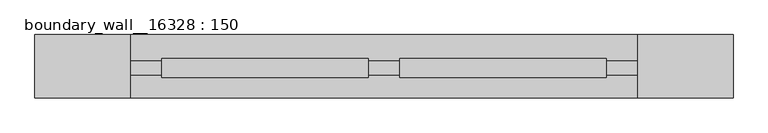
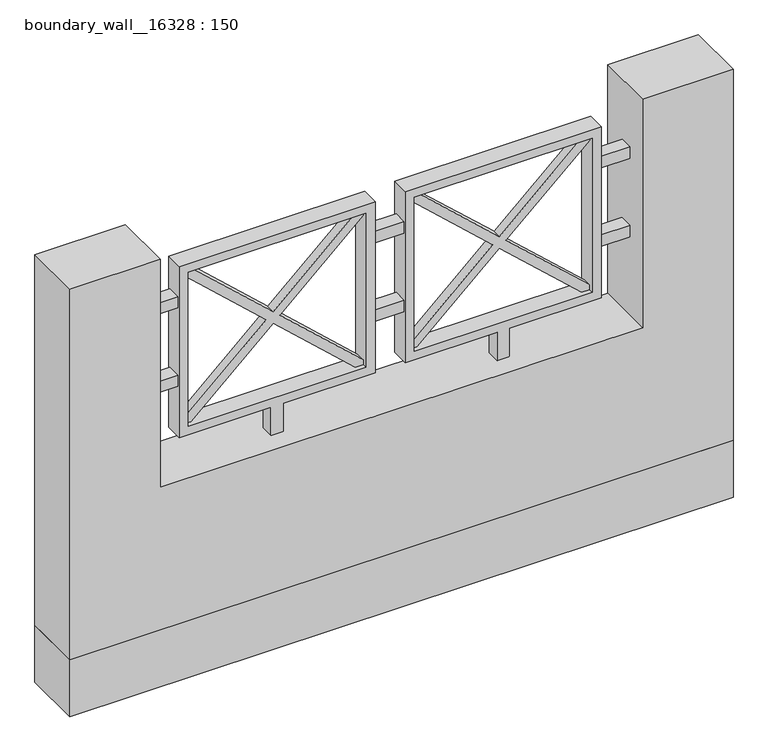
"""IFC4 building model written with IfcOpenShell, lengths in millimetres: proxy geometry, boundary_wall__16328 : 150."""

from ifc_helpers import new_model, si_unit, frame, origin, place, context, project, spatial, polyline, outline, extrude, faceted_brep, source, transform, mapped, element, save


def boundary_wall_16328_150_79515850(model_context):
    return source(origin(), model_context, "Body", "SolidModel", [
        extrude(outline(polyline([(0.0, -1100.0), (0.0, 1100.0), (1300.0, 1100.0), (1300.0, 800.0), (500.0, 800.0), (500.0, -800.0), (1300.0, -800.0), (1300.0, -1100.0), (0.0, -1100.0)])), frame((0.0, -100.0, 0.0), z_axis=(0.0, 1.0, 0.0), x_axis=(0.0, 0.0, 1.0)), (0.0, 0.0, 1.0), 200.0),
        faceted_brep([(-80.0, 10.0, 1168.1481481), (-81.6949153, 10.0, 1170.0), (-81.6949153, -20.0, 1170.0), (-80.0, -20.0, 1168.1481481), (-80.0, 10.0, 1154.08051), (-80.0, -20.0, 1154.08051), (-357.2806727, -20.0, 900.2981993), (-357.2806727, 10.0, 900.2981993), (-652.6064831, -20.0, 630.0), (-652.6064831, 10.0, 630.0), (-379.497686, 10.0, 879.9639838), (-379.497686, -20.0, 879.9639838), (-107.0405097, -20.0, 1170.0), (-379.497686, -20.0, 920.6324149), (-651.9548623, -20.0, 1170.0), (-670.0, -20.0, 1170.0), (-670.0, -20.0, 1145.8474576), (-401.7146993, -20.0, 900.2981993), (-670.0, -20.0, 654.7489411), (-670.0, -20.0, 630.0), (-106.3888889, -20.0, 630.0), (-80.0, -20.0, 630.0), (-80.0, -20.0, 646.5158887), (-107.0405097, 10.0, 1170.0), (-379.497686, 10.0, 920.6324149), (-670.0, 10.0, 654.7489411), (-401.7146993, 10.0, 900.2981993), (-80.0, 10.0, 646.5158887), (-80.0, 10.0, 630.0), (-106.3888889, 10.0, 630.0), (-670.0, 10.0, 630.0), (-670.0, 10.0, 1145.8474576), (-670.0, 10.0, 1170.0), (-651.9548623, 10.0, 1170.0), (-80.0, -35.0, 630.0), (-80.0, -35.0, 1170.0), (-80.0, 25.0, 1170.0), (-80.0, 25.0, 630.0), (-50.0, -35.0, 600.0), (-50.0, 25.0, 600.0), (-50.0, 25.0, 1200.0), (-50.0, -35.0, 1200.0), (-50.0, -27.5, 1050.0), (-50.0, -27.5, 1090.0), (-50.0, 17.5, 1090.0), (-50.0, 17.5, 1050.0), (-50.0, -27.5, 775.0), (-50.0, -27.5, 815.0), (-50.0, 17.5, 815.0), (-50.0, 17.5, 775.0), (-670.0, -35.0, 1170.0), (-670.0, 25.0, 1170.0), (-700.0, 25.0, 1200.0), (-700.0, -35.0, 1200.0), (-670.0, -35.0, 630.0), (-670.0, 25.0, 630.0), (-700.0, 25.0, 600.0), (-700.0, -35.0, 600.0), (-700.0, -27.5, 1090.0), (-700.0, -27.5, 1050.0), (-700.0, 17.5, 1050.0), (-700.0, 17.5, 1090.0), (-700.0, -27.5, 815.0), (-700.0, -27.5, 775.0), (-700.0, 17.5, 775.0), (-700.0, 17.5, 815.0), (-355.0, -35.0, 600.0), (-355.0, 10.0, 600.0), (-395.0, 10.0, 600.0), (-395.0, -35.0, 600.0), (-395.0, -35.0, 500.0), (-355.0, -35.0, 500.0), (-800.0, -27.5, 1090.0), (-800.0, -27.5, 1050.0), (-800.0, 17.5, 1050.0), (-800.0, 17.5, 1090.0), (-800.0, -27.5, 815.0), (-800.0, -27.5, 775.0), (-800.0, 17.5, 775.0), (-800.0, 17.5, 815.0), (-355.0, 10.0, 500.0), (-395.0, 10.0, 500.0), (670.0, -35.0, 630.0), (670.0, -35.0, 1170.0), (670.0, 25.0, 1170.0), (670.0, 25.0, 630.0), (670.0, 10.0, 630.0), (670.0, 10.0, 646.9396175), (670.0, -20.0, 646.9396175), (670.0, -20.0, 630.0), (670.0, 10.0, 1168.1481481), (670.0, -20.0, 1168.1481481), (670.0, -20.0, 1154.08051), (670.0, 10.0, 1154.08051), (700.0, -35.0, 600.0), (700.0, 25.0, 600.0), (700.0, 25.0, 1200.0), (700.0, -35.0, 1200.0), (700.0, -27.5, 1050.0), (700.0, -27.5, 1090.0), (700.0, 17.5, 1090.0), (700.0, 17.5, 1050.0), (700.0, -27.5, 775.0), (700.0, -27.5, 815.0), (700.0, 17.5, 815.0), (700.0, 17.5, 775.0), (80.0, -35.0, 1170.0), (80.0, -20.0, 1170.0), (98.5081006, -20.0, 1170.0), (98.5081006, 10.0, 1170.0), (80.0, 10.0, 1170.0), (80.0, 25.0, 1170.0), (668.3050847, -20.0, 1170.0), (668.3050847, 10.0, 1170.0), (642.9594903, 10.0, 1170.0), (642.9594903, -20.0, 1170.0), (50.0, 25.0, 1200.0), (50.0, -35.0, 1200.0), (80.0, -35.0, 630.0), (80.0, -20.0, 630.0), (80.0, -20.0, 654.7489411), (80.0, 10.0, 654.7489411), (80.0, 10.0, 630.0), (80.0, 25.0, 630.0), (80.0, 10.0, 1146.2711864), (80.0, -20.0, 1146.2711864), (50.0, 25.0, 600.0), (50.0, -35.0, 600.0), (50.0, -27.5, 1090.0), (50.0, -27.5, 1050.0), (50.0, 17.5, 1050.0), (50.0, 17.5, 1090.0), (50.0, -27.5, 815.0), (50.0, -27.5, 775.0), (50.0, 17.5, 775.0), (50.0, 17.5, 815.0), (644.0740741, -20.0, 630.0), (644.0740741, 10.0, 630.0), (97.3935169, 10.0, 630.0), (97.3935169, -20.0, 630.0), (395.0, -35.0, 600.0), (395.0, 10.0, 600.0), (355.0, 10.0, 600.0), (355.0, -35.0, 600.0), (355.0, -35.0, 500.0), (395.0, -35.0, 500.0), (392.9508088, -20.0, 900.5100637), (392.9508088, 10.0, 900.5100637), (370.7337955, 10.0, 880.1758482), (370.7337955, -20.0, 880.1758482), (370.7337955, -20.0, 920.8442793), (348.5167822, -20.0, 900.5100637), (370.7337955, 10.0, 920.8442793), (348.5167822, 10.0, 900.5100637), (395.0, 10.0, 500.0), (355.0, 10.0, 500.0), (800.0, -27.5, 1090.0), (800.0, -27.5, 1050.0), (800.0, 17.5, 1090.0), (800.0, 17.5, 1050.0), (800.0, -27.5, 815.0), (800.0, -27.5, 775.0), (800.0, 17.5, 815.0), (800.0, 17.5, 775.0)], [[[0, 1, 2, 3]], [[4, 5, 6, 7]], [[8, 9, 10, 11]], [[3, 2, 12, 13, 14, 15, 16, 17, 18, 19, 8, 11, 20, 21, 22, 6, 5]], [[12, 23, 24, 13]], [[25, 18, 17, 26]], [[1, 0, 4, 7, 27, 28, 29, 10, 9, 30, 25, 26, 31, 32, 33, 24, 23]], [[34, 35, 36, 37, 28, 27, 22, 21], [0, 3, 5, 4]], [[38, 39, 40, 41], [42, 43, 44, 45], [46, 47, 48, 49]], [[36, 35, 50, 15, 14, 33, 32, 51], [2, 1, 23, 12]], [[41, 40, 52, 53]], [[50, 54, 19, 18, 25, 30, 55, 51, 32, 31, 16, 15]], [[53, 52, 56, 57], [58, 59, 60, 61], [62, 63, 64, 65]], [[54, 34, 21, 20, 29, 28, 37, 55, 30, 9, 8, 19]], [[40, 39, 56, 52], [37, 36, 51, 55]], [[39, 38, 66, 67, 68, 69, 57, 56]], [[38, 41, 53, 57, 69, 70, 71, 66], [35, 34, 54, 50]], [[58, 72, 73, 59]], [[60, 74, 75, 61]], [[72, 58, 61, 75]], [[73, 72, 75, 74]], [[59, 73, 74, 60]], [[62, 76, 77, 63]], [[64, 78, 79, 65]], [[76, 62, 65, 79]], [[77, 76, 79, 78]], [[63, 77, 78, 64]], [[80, 81, 68, 67]], [[66, 71, 80, 67]], [[70, 69, 68, 81]], [[71, 70, 81, 80]], [[82, 83, 84, 85, 86, 87, 88, 89], [90, 91, 92, 93]], [[94, 95, 96, 97], [98, 99, 100, 101], [102, 103, 104, 105]], [[84, 83, 106, 107, 108, 109, 110, 111], [112, 113, 114, 115]], [[97, 96, 116, 117]], [[106, 118, 119, 120, 121, 122, 123, 111, 110, 124, 125, 107]], [[117, 116, 126, 127], [128, 129, 130, 131], [132, 133, 134, 135]], [[118, 82, 89, 136, 137, 86, 85, 123, 122, 138, 139, 119]], [[96, 95, 126, 116], [85, 84, 111, 123]], [[95, 94, 140, 141, 142, 143, 127, 126]], [[94, 97, 117, 127, 143, 144, 145, 140], [83, 82, 118, 106]], [[90, 113, 112, 91]], [[93, 92, 146, 147]], [[139, 138, 148, 149]], [[91, 112, 115, 150, 108, 107, 125, 151, 120, 119, 139, 149, 136, 89, 88, 146, 92]], [[115, 114, 152, 150]], [[121, 120, 151, 153]], [[113, 90, 93, 147, 87, 86, 137, 148, 138, 122, 121, 153, 124, 110, 109, 152, 114]], [[154, 155, 142, 141]], [[140, 145, 154, 141]], [[144, 143, 142, 155]], [[145, 144, 155, 154]], [[156, 99, 98, 157]], [[158, 159, 101, 100]], [[99, 156, 158, 100]], [[157, 98, 101, 159]], [[156, 157, 159, 158]], [[160, 103, 102, 161]], [[162, 163, 105, 104]], [[103, 160, 162, 104]], [[161, 102, 105, 163]], [[160, 161, 163, 162]], [[128, 43, 42, 129]], [[130, 45, 44, 131]], [[43, 128, 131, 44]], [[129, 42, 45, 130]], [[132, 47, 46, 133]], [[134, 49, 48, 135]], [[47, 132, 135, 48]], [[133, 46, 49, 134]], [[27, 7, 6, 22]], [[24, 33, 14, 13]], [[17, 16, 31, 26]], [[20, 11, 10, 29]], [[148, 137, 136, 149]], [[124, 153, 151, 125]], [[87, 147, 146, 88]], [[152, 109, 108, 150]]]),
        extrude(outline(polyline([(1100.0, -100.0), (-1100.0, -100.0), (-1100.0, 100.0), (1100.0, 100.0), (1100.0, -100.0)])), frame((0.0, 0.0, -200.0), z_axis=(0.0, 0.0, 1.0), x_axis=(1.0, 0.0, 0.0)), (0.0, 0.0, 1.0), 200.0),
    ])


if __name__ == "__main__":
    model = new_model("IFC4")
    model_context = context("Model", 3, world=origin())
    ifc_project = project(units=[si_unit("LENGTHUNIT", "METRE", prefix="MILLI")], contexts=[model_context])
    site = spatial("IfcSite", under=ifc_project)
    building = spatial("IfcBuilding", under=site)
    placement = place(None, origin())
    boundary_wall_16328_150_shape = boundary_wall_16328_150_79515850(model_context)
    element("IfcBuildingElementProxy", 1, Name="boundary_wall__16328 : 150", ObjectType="boundary_wall__16328 : 150", at=placement, inside=building, context=model_context, shape_type="MappedRepresentation", body=[
        mapped(boundary_wall_16328_150_shape, transform((0.0, 0.0, 0.0), x_axis=(1.0, 0.0, 0.0), y_axis=(0.0, 1.0, 0.0), z_axis=(0.0, 0.0, 1.0))),
    ])
    save(model, "model.ifc")

# Revit data of these elements
# Type "boundary_wall__16328 : 150"
#   Wight Hand 2 = 0' - 11.81102"
#   Wight Hand 1 = 0' - 11.81102"
#   Void Wight = 5' - 2.99213"
#   Top.High = 2' - 7.49606"
#   F.base = 0' - 3.93701"
#   F.Wight 2 = 2' - 1.59055"
#   F.Wight 1 = 2' - 1.59055"
#   F.R = 0' - 3.93701"
#   F.L = 0' - 3.93701"
#   F.High = 1' - 11.62205"
#   Bace.High = 1' - 7.68504"
#   Default Elevation = 0
# Element 1 (IfcBuildingElementProxy, "boundary_wall__16328 : 150")
#   Materials on its faces: "Metal"
# Materials
#   "Metal": class "Generic", colour RGB 65 64 62, transparency 0, Cost = 0
